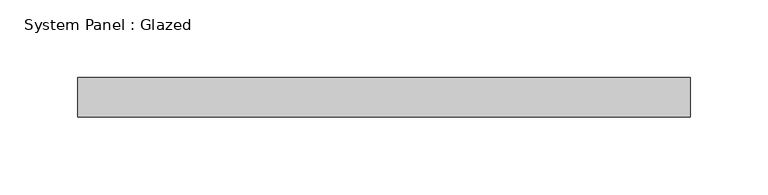
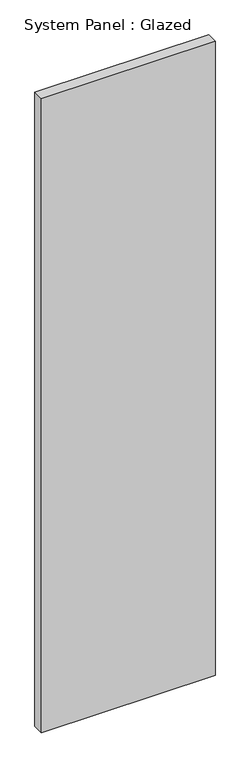
"""IFC4 building model written with IfcOpenShell, lengths in millimetres: plate geometry, System Panel : Glazed."""

from ifc_helpers import new_model, si_unit, origin, origin_with_axes, place, context, project, spatial, polyline, outline, extrude, source, transform, mapped, element, save


def system_panel_glazed_f4403250(model_context):
    return source(origin(), model_context, "Body", "SweptSolid", [
        extrude(outline(polyline([(196.85, 19.05), (-196.85, 19.05), (-196.85, 44.45), (196.85, 44.45), (196.85, 19.05)])), origin_with_axes(), (0.0, 0.0, 1.0), 1519.9538703),
    ])


if __name__ == "__main__":
    model = new_model("IFC4")
    model_context = context("Model", 3, world=origin())
    ifc_project = project(units=[si_unit("LENGTHUNIT", "METRE", prefix="MILLI")], contexts=[model_context])
    site = spatial("IfcSite", under=ifc_project)
    building = spatial("IfcBuilding", under=site)
    placement = place(None, origin())
    system_panel_glazed_shape = system_panel_glazed_f4403250(model_context)
    element("IfcPlate", 1, ObjectType="System Panel : Glazed", at=placement, inside=building, context=model_context, shape_type="MappedRepresentation", body=[
        mapped(system_panel_glazed_shape, transform((0.0, 0.0, 0.0), x_axis=(1.0, 0.0, 0.0), y_axis=(0.0, 1.0, 0.0), z_axis=(0.0, 0.0, 1.0))),
    ])
    save(model, "model.ifc")

# Revit data of these elements
# Type "System Panel : Glazed"
#   Construction Type Id = "GSP4R"
#   Analytic Construction = "1/8 in Pilkington single glazing"
#   Visual Light Transmittance = 0.9
#   Solar Heat Gain Coefficient = 0.86
#   Heat Transfer Coefficient (U) = 1.18115 BTU/(h·ft²·°F)
#   Define Thermal Properties by = 1
# Element 1 (IfcPlate, "System Panel : Glazed")
#   Materials on its faces: "Glass"
# Materials
#   "Glass": class "Glass", colour RGB 0 128 192, transparency 0.75, Description = "Soda Lime Glass", Cost = 0
